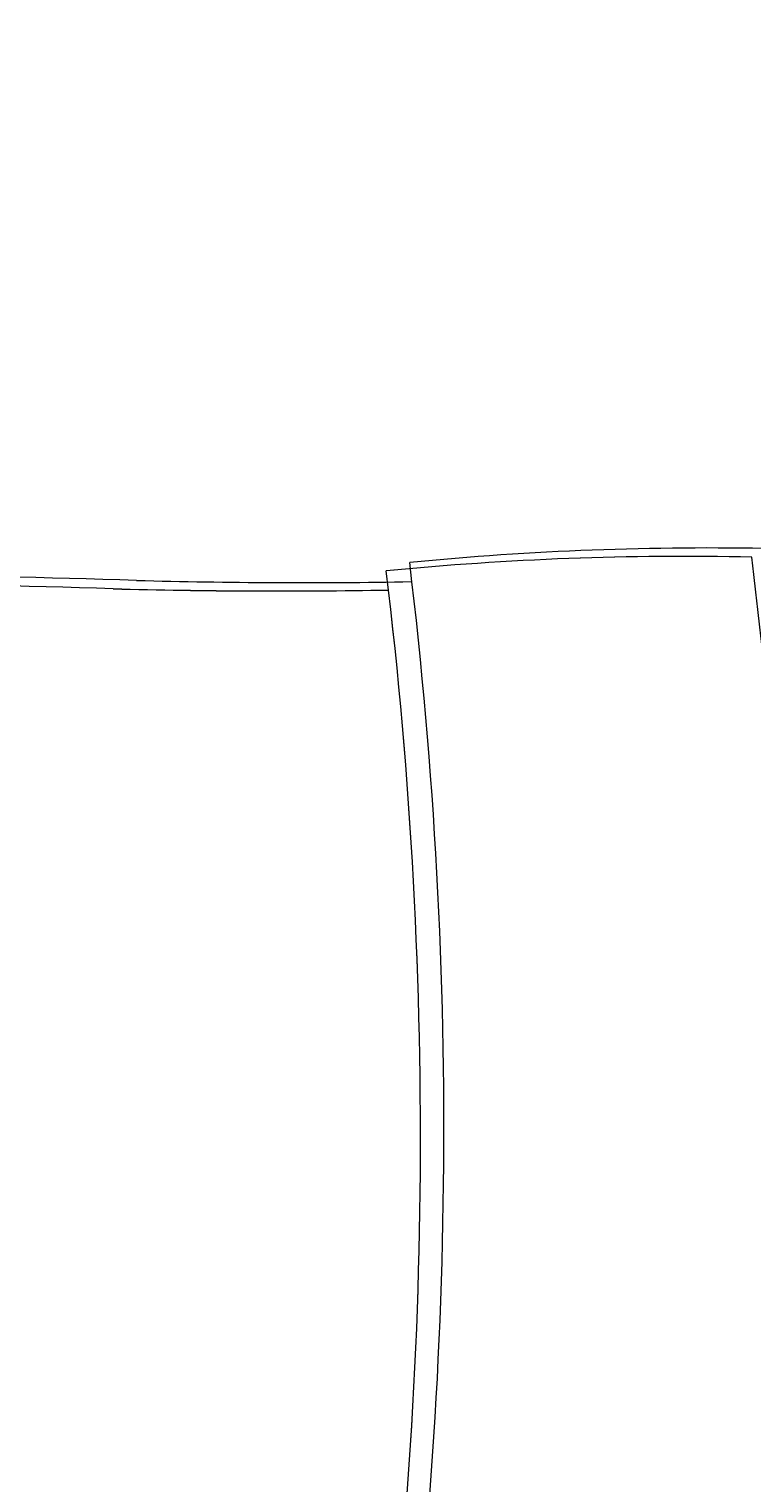
# Model space of a CAD drawing. Units: inches. Extents: x 1962 to 2771, y 1245 to 2660.
# Tile 76 of 114: x 2626 to 2641, y 2051 to 2082. Entities that reach past the tile are written whole.
import ezdxf

# ---------------------------------------------------------------- set-up
doc = ezdxf.new("R2010")
doc.units = ezdxf.units.IN
doc.layers.add('A-ANNO-DIMS', color=2, linetype='Continuous', lineweight=18)
doc.layers.add('A-FURN', color=8, linetype='Continuous', lineweight=13)
doc.styles.get("Standard").update_dxf_attribs({"font": 'arial.ttf'})
doc.dimstyles.get("Standard").update_dxf_attribs({"dimtxt": 0.18, "dimasz": 0.18, "dimexe": 0.18, "dimexo": 0.0625, "dimgap": 0.09, "dimtad": 0, "dimtih": 1, "dimtoh": 1, "dimdec": 4, "dimzin": 0, "dimdsep": 46, "dimtxsty": 'Standard', "dimcen": 0.09, "dimadec": 0, "dimazin": 0, "dimtfac": 1, "dimtdec": 4, "dimtofl": 0, "dimtmove": 0, "dimatfit": 3, "dimfxl": 1, "dimtolj": 1, "dimtzin": 0, "dimarcsym": 0})

# ---------------------------------------------------------------- blocks, each defined once
blk = doc.blocks.new('BED-PLAN')
for centre, radius, start, end in [((124.254, 14.115), 102.556, 171.78449, 186.90062), ((124.254, 14.115), 102.556, 171.78449, 186.90062), ((124.762, 14.297), 102.556, 171.78449, 186.90062), ((124.762, 14.296), 102.556, 171.78449, 186.90062), ((145.219, 17.161), 131.131, 176.08655, 186.78213), ((24.78, -132.989), 135.218, 88.4762, 91.00819), ((24.78, -132.989), 135.218, 88.4762, 91.00819), ((25.288, -132.807), 135.218, 88.4762, 91.00819), ((25.288, -132.808), 135.218, 88.4762, 91.00819), ((40.74, 385.562), 383.382, 268.22771, 271.71854), ((40.74, 385.561), 383.382, 268.22771, 271.71854), ((16.482, 67.877), 66.218, 268.72178, 275.60397), ((16.483, 67.877), 66.218, 268.72178, 275.60397), ((40.232, 385.38), 383.382, 268.22771, 271.71854), ((40.232, 385.38), 383.382, 268.22771, 271.71854), ((15.974, 67.695), 66.218, 268.72178, 275.60397), ((15.974, 67.695), 66.218, 268.72178, 275.60397)]:
    blk.add_arc(centre, radius, start, end)
blk = doc.blocks.new('*D40')
at = {"layer": 'A-ANNO-DIMS', "color": 0, "lineweight": -2, "transparency": 16777216}
for p, q in [((2072.02, 2033.906), (2072.02, 2583.474)), ((2072.2, 2583.294), (2366.02, 2583.294)), ((2660.627, 2583.294), (2366.808, 2583.294)), ((2660.807, 2524.406), (2660.807, 2583.474))]:
    blk.add_line(p, q, dxfattribs=at)
at = {"layer": 'A-ANNO-DIMS', "color": 0, "transparency": 16777216}
for points in [[(2072.2, 2583.324), (2072.2, 2583.264), (2072.02, 2583.294)], [(2660.627, 2583.324), (2660.627, 2583.264), (2660.807, 2583.294)]]:
    blk.add_solid(points, dxfattribs=at)
at = {"layer": 'Defpoints', "color": 0, "transparency": 16777216}
for p in [(2660.807, 2583.294), (2660.807, 2524.344), (2072.02, 2033.844)]:
    blk.add_point(p, dxfattribs=at)
at = {"layer": 'A-ANNO-DIMS', "color": 0, "transparency": 16777216, "insert": (2366.414, 2583.294), "char_height": 0.18, "attachment_point": 5}
blk.add_mtext('\\A1;588.8', dxfattribs=at)

msp = doc.modelspace()

# ---------------------------------------------------------------- block references
at = {"layer": 'A-FURN', "rotation": 180}
msp.add_blockref('BED-PLAN', (2656.3074, 2072.498), dxfattribs=at)

# ---------------------------------------------------------------- dimensions: what is measured, and where the dimension line sits
at = {"layer": 'A-ANNO-DIMS'}
dim = msp.add_linear_dim(base=(2660.8074, 2583.2937), p1=(2072.0204, 2033.8437), p2=(2660.8074, 2524.3437), dimstyle='Standard', override={"dimdec": 1, "dimlfac": 1, "dimrnd": 0, "dimzin": 0, "dimdsep": 46, "dimlunit": 2}, dxfattribs=at)
dim.commit()
dim.dimension.update_dxf_attribs({"geometry": '*D40', "text_midpoint": (2366.4139, 2583.2937)})

doc.saveas('drawing.dxf')
